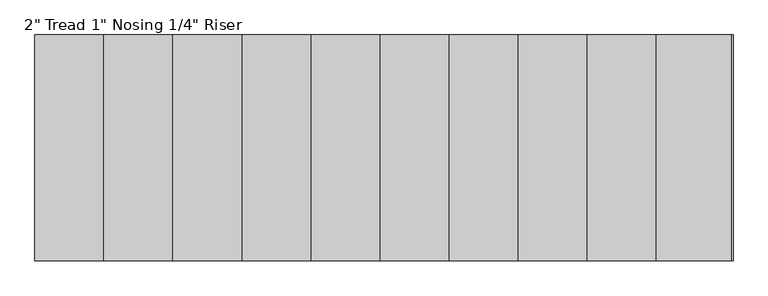
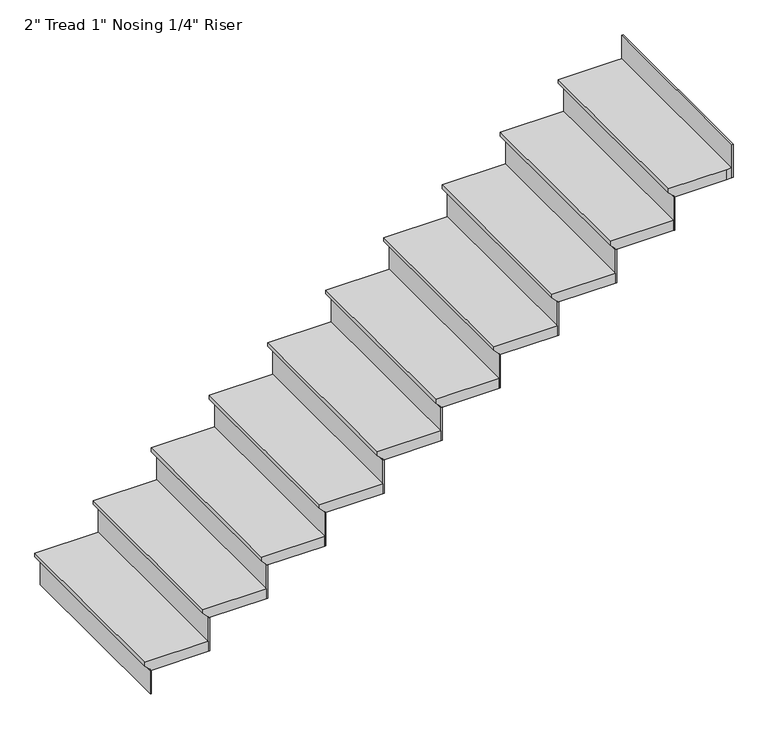
"""IFC4 building model written with IfcOpenShell, lengths in millimetres: stair flight geometry."""

from ifc_helpers import new_model, si_unit, origin, place, context, project, spatial, faceted_brep, source, transform, mapped, element, save


def stair_flight_bde5577f(model_context):
    return source(origin(), model_context, "Body", "Brep", [
        faceted_brep([(-9709.3703437, -6347.7504041, 3198.2833333), (-9709.3703437, -6347.7504041, 3217.3333333), (-9709.3703437, -5433.3504041, 3217.3333333), (-9709.3703437, -5433.3504041, 3198.2833333), (-9683.9703437, -6347.7504041, 3172.8833333), (-9683.9703437, -5433.3504041, 3172.8833333), (-9404.5703437, -6347.7504041, 3217.3333333), (-9404.5703437, -5433.3504041, 3217.3333333), (-9683.9703437, -5433.3504041, 3166.5333333), (-9404.5703437, -5433.3504041, 3166.5333333), (-9404.5703437, -6347.7504041, 3166.5333333), (-9683.9703437, -6347.7504041, 3166.5333333)], [[[0, 1, 2, 3]], [[4, 0, 3, 5]], [[2, 1, 6, 7]], [[8, 9, 10, 11]], [[2, 7, 9, 8, 5, 3]], [[8, 11, 4, 5]], [[6, 1, 0, 4, 11, 10]], [[7, 6, 10, 9]]]),
        faceted_brep([(-9683.9703437, -6347.7504041, 3166.5333333), (-9683.9703437, -6347.7504041, 3048.0), (-9677.6203437, -6347.7504041, 3048.0), (-9677.6203437, -6347.7504041, 3166.5333333), (-9683.9703437, -5433.3504041, 3166.5333333), (-9677.6203437, -5433.3504041, 3166.5333333), (-9677.6203437, -5433.3504041, 3048.0), (-9683.9703437, -5433.3504041, 3048.0)], [[[0, 1, 2, 3]], [[4, 5, 6, 7]], [[1, 0, 4, 7]], [[2, 1, 7, 6]], [[3, 2, 6, 5]], [[0, 3, 5, 4]]]),
        faceted_brep([(-9404.5703437, -6347.7504041, 3335.8666667), (-9404.5703437, -6347.7504041, 3166.5333333), (-9398.2203437, -6347.7504041, 3166.5333333), (-9398.2203437, -6347.7504041, 3335.8666667), (-9404.5703437, -5433.3504041, 3335.8666667), (-9398.2203437, -5433.3504041, 3335.8666667), (-9398.2203437, -5433.3504041, 3166.5333333), (-9404.5703437, -5433.3504041, 3166.5333333)], [[[0, 1, 2, 3]], [[4, 5, 6, 7]], [[1, 0, 4, 7]], [[2, 1, 7, 6]], [[3, 2, 6, 5]], [[0, 3, 5, 4]]]),
        faceted_brep([(-9429.9703437, -5433.3504041, 3386.6666667), (-9429.9703437, -6347.7504041, 3386.6666667), (-9125.1703437, -6347.7504041, 3386.6666667), (-9125.1703437, -5433.3504041, 3386.6666667), (-9404.5703437, -5433.3504041, 3335.8666667), (-9125.1703437, -5433.3504041, 3335.8666667), (-9125.1703437, -6347.7504041, 3335.8666667), (-9404.5703437, -6347.7504041, 3335.8666667), (-9404.5703437, -5433.3504041, 3342.2166667), (-9429.9703437, -5433.3504041, 3367.6166667), (-9404.5703437, -6347.7504041, 3342.2166667), (-9429.9703437, -6347.7504041, 3367.6166667)], [[[0, 1, 2, 3]], [[4, 5, 6, 7]], [[0, 3, 5, 4, 8, 9]], [[4, 7, 10, 8]], [[2, 1, 11, 10, 7, 6]], [[3, 2, 6, 5]], [[11, 1, 0, 9]], [[10, 11, 9, 8]]]),
        faceted_brep([(-9125.1703437, -6347.7504041, 3505.2), (-9125.1703437, -6347.7504041, 3335.8666667), (-9118.8203437, -6347.7504041, 3335.8666667), (-9118.8203437, -6347.7504041, 3505.2), (-9125.1703437, -5433.3504041, 3505.2), (-9118.8203437, -5433.3504041, 3505.2), (-9118.8203437, -5433.3504041, 3335.8666667), (-9125.1703437, -5433.3504041, 3335.8666667)], [[[0, 1, 2, 3]], [[4, 5, 6, 7]], [[1, 0, 4, 7]], [[2, 1, 7, 6]], [[3, 2, 6, 5]], [[0, 3, 5, 4]]]),
        faceted_brep([(-9150.5703437, -5433.3504041, 3556.0), (-9150.5703437, -6347.7504041, 3556.0), (-8845.7703437, -6347.7504041, 3556.0), (-8845.7703437, -5433.3504041, 3556.0), (-9125.1703437, -5433.3504041, 3505.2), (-8845.7703437, -5433.3504041, 3505.2), (-8845.7703437, -6347.7504041, 3505.2), (-9125.1703437, -6347.7504041, 3505.2), (-9125.1703437, -5433.3504041, 3511.55), (-9150.5703437, -5433.3504041, 3536.95), (-9125.1703437, -6347.7504041, 3511.55), (-9150.5703437, -6347.7504041, 3536.95)], [[[0, 1, 2, 3]], [[4, 5, 6, 7]], [[0, 3, 5, 4, 8, 9]], [[4, 7, 10, 8]], [[2, 1, 11, 10, 7, 6]], [[3, 2, 6, 5]], [[11, 1, 0, 9]], [[10, 11, 9, 8]]]),
        faceted_brep([(-8845.7703437, -6347.7504041, 3674.5333333), (-8845.7703437, -6347.7504041, 3505.2), (-8839.4203437, -6347.7504041, 3505.2), (-8839.4203437, -6347.7504041, 3674.5333333), (-8845.7703437, -5433.3504041, 3674.5333333), (-8839.4203437, -5433.3504041, 3674.5333333), (-8839.4203437, -5433.3504041, 3505.2), (-8845.7703437, -5433.3504041, 3505.2)], [[[0, 1, 2, 3]], [[4, 5, 6, 7]], [[1, 0, 4, 7]], [[2, 1, 7, 6]], [[3, 2, 6, 5]], [[0, 3, 5, 4]]]),
        faceted_brep([(-8871.1703437, -5433.3504041, 3725.3333333), (-8871.1703437, -6347.7504041, 3725.3333333), (-8566.3703437, -6347.7504041, 3725.3333333), (-8566.3703437, -5433.3504041, 3725.3333333), (-8845.7703437, -5433.3504041, 3674.5333333), (-8566.3703437, -5433.3504041, 3674.5333333), (-8566.3703437, -6347.7504041, 3674.5333333), (-8845.7703437, -6347.7504041, 3674.5333333), (-8845.7703437, -5433.3504041, 3680.8833333), (-8871.1703437, -5433.3504041, 3706.2833333), (-8845.7703437, -6347.7504041, 3680.8833333), (-8871.1703437, -6347.7504041, 3706.2833333)], [[[0, 1, 2, 3]], [[4, 5, 6, 7]], [[0, 3, 5, 4, 8, 9]], [[4, 7, 10, 8]], [[2, 1, 11, 10, 7, 6]], [[3, 2, 6, 5]], [[11, 1, 0, 9]], [[10, 11, 9, 8]]]),
        faceted_brep([(-8566.3703437, -6347.7504041, 3843.8666667), (-8566.3703437, -6347.7504041, 3674.5333333), (-8560.0203437, -6347.7504041, 3674.5333333), (-8560.0203437, -6347.7504041, 3843.8666667), (-8566.3703437, -5433.3504041, 3843.8666667), (-8560.0203437, -5433.3504041, 3843.8666667), (-8560.0203437, -5433.3504041, 3674.5333333), (-8566.3703437, -5433.3504041, 3674.5333333)], [[[0, 1, 2, 3]], [[4, 5, 6, 7]], [[1, 0, 4, 7]], [[2, 1, 7, 6]], [[3, 2, 6, 5]], [[0, 3, 5, 4]]]),
        faceted_brep([(-8591.7703437, -5433.3504041, 3894.6666667), (-8591.7703437, -6347.7504041, 3894.6666667), (-8286.9703437, -6347.7504041, 3894.6666667), (-8286.9703437, -5433.3504041, 3894.6666667), (-8566.3703437, -5433.3504041, 3843.8666667), (-8286.9703437, -5433.3504041, 3843.8666667), (-8286.9703437, -6347.7504041, 3843.8666667), (-8566.3703437, -6347.7504041, 3843.8666667), (-8566.3703437, -5433.3504041, 3850.2166667), (-8591.7703437, -5433.3504041, 3875.6166667), (-8566.3703437, -6347.7504041, 3850.2166667), (-8591.7703437, -6347.7504041, 3875.6166667)], [[[0, 1, 2, 3]], [[4, 5, 6, 7]], [[0, 3, 5, 4, 8, 9]], [[4, 7, 10, 8]], [[2, 1, 11, 10, 7, 6]], [[3, 2, 6, 5]], [[11, 1, 0, 9]], [[10, 11, 9, 8]]]),
        faceted_brep([(-8286.9703437, -6347.7504041, 4013.2), (-8286.9703437, -6347.7504041, 3843.8666667), (-8280.6203437, -6347.7504041, 3843.8666667), (-8280.6203437, -6347.7504041, 4013.2), (-8286.9703437, -5433.3504041, 4013.2), (-8280.6203437, -5433.3504041, 4013.2), (-8280.6203437, -5433.3504041, 3843.8666667), (-8286.9703437, -5433.3504041, 3843.8666667)], [[[0, 1, 2, 3]], [[4, 5, 6, 7]], [[1, 0, 4, 7]], [[2, 1, 7, 6]], [[3, 2, 6, 5]], [[0, 3, 5, 4]]]),
        faceted_brep([(-8312.3703437, -5433.3504041, 4064.0), (-8312.3703437, -6347.7504041, 4064.0), (-8007.5703437, -6347.7504041, 4064.0), (-8007.5703437, -5433.3504041, 4064.0), (-8286.9703437, -5433.3504041, 4013.2), (-8007.5703437, -5433.3504041, 4013.2), (-8007.5703437, -6347.7504041, 4013.2), (-8286.9703437, -6347.7504041, 4013.2), (-8286.9703437, -5433.3504041, 4019.55), (-8312.3703437, -5433.3504041, 4044.95), (-8286.9703437, -6347.7504041, 4019.55), (-8312.3703437, -6347.7504041, 4044.95)], [[[0, 1, 2, 3]], [[4, 5, 6, 7]], [[0, 3, 5, 4, 8, 9]], [[4, 7, 10, 8]], [[2, 1, 11, 10, 7, 6]], [[3, 2, 6, 5]], [[11, 1, 0, 9]], [[10, 11, 9, 8]]]),
        faceted_brep([(-8007.5703437, -6347.7504041, 4182.5333333), (-8007.5703437, -6347.7504041, 4013.2), (-8001.2203437, -6347.7504041, 4013.2), (-8001.2203437, -6347.7504041, 4182.5333333), (-8007.5703437, -5433.3504041, 4182.5333333), (-8001.2203437, -5433.3504041, 4182.5333333), (-8001.2203437, -5433.3504041, 4013.2), (-8007.5703437, -5433.3504041, 4013.2)], [[[0, 1, 2, 3]], [[4, 5, 6, 7]], [[1, 0, 4, 7]], [[2, 1, 7, 6]], [[3, 2, 6, 5]], [[0, 3, 5, 4]]]),
        faceted_brep([(-8032.9703437, -5433.3504041, 4233.3333333), (-8032.9703437, -6347.7504041, 4233.3333333), (-7728.1703437, -6347.7504041, 4233.3333333), (-7728.1703437, -5433.3504041, 4233.3333333), (-8007.5703437, -5433.3504041, 4182.5333333), (-7728.1703437, -5433.3504041, 4182.5333333), (-7728.1703437, -6347.7504041, 4182.5333333), (-8007.5703437, -6347.7504041, 4182.5333333), (-8007.5703437, -5433.3504041, 4188.8833333), (-8032.9703437, -5433.3504041, 4214.2833333), (-8007.5703437, -6347.7504041, 4188.8833333), (-8032.9703437, -6347.7504041, 4214.2833333)], [[[0, 1, 2, 3]], [[4, 5, 6, 7]], [[0, 3, 5, 4, 8, 9]], [[4, 7, 10, 8]], [[2, 1, 11, 10, 7, 6]], [[3, 2, 6, 5]], [[11, 1, 0, 9]], [[10, 11, 9, 8]]]),
        faceted_brep([(-7728.1703437, -6347.7504041, 4351.8666667), (-7728.1703437, -6347.7504041, 4182.5333333), (-7721.8203437, -6347.7504041, 4182.5333333), (-7721.8203437, -6347.7504041, 4351.8666667), (-7728.1703437, -5433.3504041, 4351.8666667), (-7721.8203437, -5433.3504041, 4351.8666667), (-7721.8203437, -5433.3504041, 4182.5333333), (-7728.1703437, -5433.3504041, 4182.5333333)], [[[0, 1, 2, 3]], [[4, 5, 6, 7]], [[1, 0, 4, 7]], [[2, 1, 7, 6]], [[3, 2, 6, 5]], [[0, 3, 5, 4]]]),
        faceted_brep([(-7753.5703437, -5433.3504041, 4402.6666667), (-7753.5703437, -6347.7504041, 4402.6666667), (-7448.7703437, -6347.7504041, 4402.6666667), (-7448.7703437, -5433.3504041, 4402.6666667), (-7728.1703437, -5433.3504041, 4351.8666667), (-7448.7703437, -5433.3504041, 4351.8666667), (-7448.7703437, -6347.7504041, 4351.8666667), (-7728.1703437, -6347.7504041, 4351.8666667), (-7728.1703437, -5433.3504041, 4358.2166667), (-7753.5703437, -5433.3504041, 4383.6166667), (-7728.1703437, -6347.7504041, 4358.2166667), (-7753.5703437, -6347.7504041, 4383.6166667)], [[[0, 1, 2, 3]], [[4, 5, 6, 7]], [[0, 3, 5, 4, 8, 9]], [[4, 7, 10, 8]], [[2, 1, 11, 10, 7, 6]], [[3, 2, 6, 5]], [[11, 1, 0, 9]], [[10, 11, 9, 8]]]),
        faceted_brep([(-7448.7703437, -6347.7504041, 4521.2), (-7448.7703437, -6347.7504041, 4351.8666667), (-7442.4203437, -6347.7504041, 4351.8666667), (-7442.4203437, -6347.7504041, 4521.2), (-7448.7703437, -5433.3504041, 4521.2), (-7442.4203437, -5433.3504041, 4521.2), (-7442.4203437, -5433.3504041, 4351.8666667), (-7448.7703437, -5433.3504041, 4351.8666667)], [[[0, 1, 2, 3]], [[4, 5, 6, 7]], [[1, 0, 4, 7]], [[2, 1, 7, 6]], [[3, 2, 6, 5]], [[0, 3, 5, 4]]]),
        faceted_brep([(-7474.1703437, -5433.3504041, 4572.0), (-7474.1703437, -6347.7504041, 4572.0), (-7169.3703437, -6347.7504041, 4572.0), (-7169.3703437, -5433.3504041, 4572.0), (-7448.7703437, -5433.3504041, 4521.2), (-7169.3703437, -5433.3504041, 4521.2), (-7169.3703437, -6347.7504041, 4521.2), (-7448.7703437, -6347.7504041, 4521.2), (-7448.7703437, -5433.3504041, 4527.55), (-7474.1703437, -5433.3504041, 4552.95), (-7448.7703437, -6347.7504041, 4527.55), (-7474.1703437, -6347.7504041, 4552.95)], [[[0, 1, 2, 3]], [[4, 5, 6, 7]], [[0, 3, 5, 4, 8, 9]], [[4, 7, 10, 8]], [[2, 1, 11, 10, 7, 6]], [[3, 2, 6, 5]], [[11, 1, 0, 9]], [[10, 11, 9, 8]]]),
        faceted_brep([(-6889.9703437, -6347.7504041, 4859.8666667), (-6889.9703437, -6347.7504041, 4690.5333333), (-6883.6203437, -6347.7504041, 4690.5333333), (-6883.6203437, -6347.7504041, 4859.8666667), (-6889.9703437, -5433.3504041, 4859.8666667), (-6883.6203437, -5433.3504041, 4859.8666667), (-6883.6203437, -5433.3504041, 4690.5333333), (-6889.9703437, -5433.3504041, 4690.5333333)], [[[0, 1, 2, 3]], [[4, 5, 6, 7]], [[1, 0, 4, 7]], [[2, 1, 7, 6]], [[3, 2, 6, 5]], [[0, 3, 5, 4]]]),
        faceted_brep([(-7169.3703437, -6347.7504041, 4690.5333333), (-7169.3703437, -6347.7504041, 4521.2), (-7163.0203437, -6347.7504041, 4521.2), (-7163.0203437, -6347.7504041, 4690.5333333), (-7169.3703437, -5433.3504041, 4690.5333333), (-7163.0203437, -5433.3504041, 4690.5333333), (-7163.0203437, -5433.3504041, 4521.2), (-7169.3703437, -5433.3504041, 4521.2)], [[[0, 1, 2, 3]], [[4, 5, 6, 7]], [[1, 0, 4, 7]], [[2, 1, 7, 6]], [[3, 2, 6, 5]], [[0, 3, 5, 4]]]),
        faceted_brep([(-6889.9703437, -5433.3504041, 4741.3333333), (-6915.3703437, -5433.3504041, 4741.3333333), (-7194.7703437, -5433.3504041, 4741.3333333), (-7194.7703437, -6347.7504041, 4741.3333333), (-6915.3703437, -6347.7504041, 4741.3333333), (-6889.9703437, -6347.7504041, 4741.3333333), (-6915.3703437, -5433.3504041, 4690.5333333), (-6889.9703437, -5433.3504041, 4690.5333333), (-6889.9703437, -6347.7504041, 4690.5333333), (-6915.3703437, -6347.7504041, 4690.5333333), (-7169.3703437, -6347.7504041, 4690.5333333), (-7169.3703437, -5433.3504041, 4690.5333333), (-7169.3703437, -5433.3504041, 4696.8833333), (-7194.7703437, -5433.3504041, 4722.2833333), (-7169.3703437, -6347.7504041, 4696.8833333), (-7194.7703437, -6347.7504041, 4722.2833333)], [[[0, 1, 2, 3, 4, 5]], [[6, 7, 8, 9, 10, 11]], [[1, 0, 7, 6]], [[2, 1, 6, 11, 12, 13]], [[11, 10, 14, 12]], [[4, 3, 15, 14, 10, 9]], [[5, 4, 9, 8]], [[0, 5, 8, 7]], [[15, 3, 2, 13]], [[14, 15, 13, 12]]]),
    ])


if __name__ == "__main__":
    model = new_model("IFC4")
    model_context = context("Model", 3, world=origin())
    ifc_project = project(units=[si_unit("LENGTHUNIT", "METRE", prefix="MILLI")], contexts=[model_context])
    site = spatial("IfcSite", under=ifc_project)
    building = spatial("IfcBuilding", under=site)
    placement = place(None, origin())
    stair_flight_shape = stair_flight_bde5577f(model_context)
    element("IfcStairFlight", 1, ObjectType="2\" Tread 1\" Nosing 1/4\" Riser", at=placement, inside=building, context=model_context, shape_type="MappedRepresentation", body=[
        mapped(stair_flight_shape, transform((0.0, 0.0, 0.0), x_axis=(1.0, 0.0, 0.0), y_axis=(0.0, 1.0, 0.0), z_axis=(0.0, 0.0, 1.0))),
    ])
    save(model, "model.ifc")
